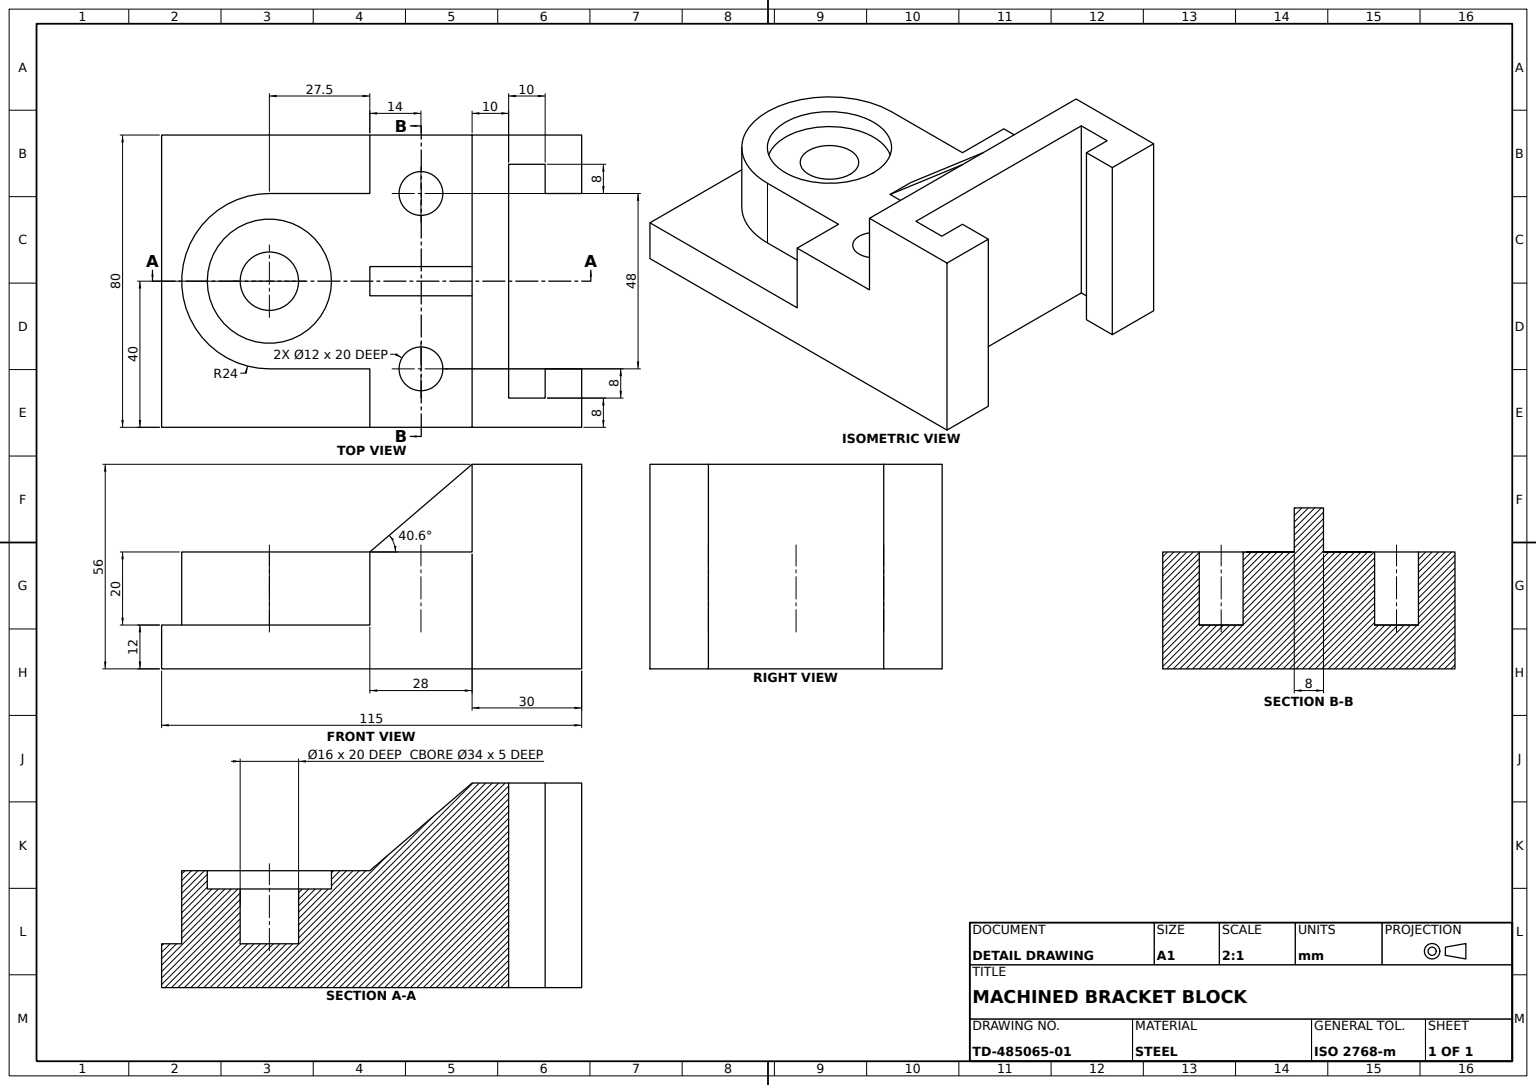
SolidWorks part; units mm, degrees
material "Plain Carbon Steel"
ref_plane "Front Plane" through (0, 0, 0) normal (0, 0, 1) x (1, 0, 0)
ref_plane "Top Plane" through (0, 0, 0) normal (0, 1, 0) x (1, 0, 0)
ref_plane "Right Plane" through (0, 0, 0) normal (1, 0, 0) x (0, 0, -1)
sketch "Base Plate Sketch" plane through (0, 0, 0) normal (0, 1, 0) x (1, 0, 0)
  line L1 (-40, -57.5) -> (40, -57.5)
  line L2 (-40, -57.5) -> (-40, 57.5)
  line L3 (-40, 57.5) -> (40, 57.5)
  line L4 (40, -57.5) -> (40, 57.5)
  line L5 (-40, -57.5) -> (40, 57.5) construction
  line L6 (-40, 57.5) -> (40, -57.5) construction
  point P0 (0, 0)
  dimension "D1" = 115
  dimension "D2" = 80
extrude "Base Plate" add sketch "Base Plate Sketch" along normal blind 12
sketch "Back Wall Sketch" plane through (0, 12, 0) normal (0, 1, 0) x (1, 0, 0)
  line L0 (40, -57.5) -> (40, 57.5) construction
  line L1 (-40, 57.5) -> (40, 57.5)
  line L2 (-40, 57.5) -> (-40, 27.5)
  line L3 (-40, 27.5) -> (40, 27.5)
  line L4 (40, 57.5) -> (40, 27.5)
  dimension "D1" = 30
extrude "Back Wall" add sketch "Back Wall Sketch" along normal blind 44
sketch "Wall Slot Sketch" plane through (0, 56, 0) normal (0, 1, 0) x (1, 0, 0)
  line L0 (-24, 57.5) -> (-24, 47.5)
  line L1 (40, 57.5) -> (-40, 57.5) construction
  line L2 (-24, 47.5) -> (-32, 47.5)
  line L3 (-32, 47.5) -> (-32, 37.5)
  line L4 (-32, 37.5) -> (32, 37.5)
  line L5 (32, 37.5) -> (32, 47.5)
  line L6 (32, 47.5) -> (24, 47.5)
  line L7 (24, 47.5) -> (24, 57.5)
  line L8 (24, 57.5) -> (-24, 57.5)
  dimension "D1" = 16
  dimension "D2" = 16
  dimension "D3" = 10
  dimension "D4" = 10
  dimension "D5" = 8
  dimension "D6" = 8
  dimension "D7" = 10
extrude "Wall Slot Cut" cut sketch "Wall Slot Sketch" against normal through all
sketch "Boss Pad Sketch" plane through (0, 12, 0) normal (0, 1, 0) x (1, 0, 0)
  line L0 (40, -57.5) -> (40, 27.5) construction
  line L1 (-40, 27.5) -> (40, 27.5)
  line L2 (-40, 27.5) -> (-40, -0.5)
  line L3 (-40, -0.5) -> (-24, -0.5)
  line L4 (40, 27.5) -> (40, -0.5)
  line L5 (-24, -28) -> (-24, -0.5)
  line L6 (24, -28) -> (24, -0.5)
  line L7 (24, -0.5) -> (40, -0.5)
  arc A0 (-24, -28) -> (24, -28) centre (0, -28) ccw
  circle A1 centre (-24, 13.5) radius 6
  circle A2 centre (24, 13.5) radius 6
  dimension "D2" = 48
  dimension "D5" = 12
  dimension "D6" = 12
  dimension "D1" = 28
  dimension "D3" = 28
  dimension "D4" = 27.5
  dimension "D7" = 14
  dimension "D8" = 16
  dimension "D9" = 14
  dimension "D10" = 16
extrude "Boss Pad" add sketch "Boss Pad Sketch" along normal blind 20
sketch "Counterbore Sketch" plane through (0, 32, 0) normal (0, 1, 0) x (1, 0, 0)
  circle A0 centre (0, -28) radius 17
  dimension "D1" = 34
extrude "Counterbore Ø34x5" cut sketch "Counterbore Sketch" against normal blind 5
sketch "Bore Sketch" plane through (0, 27, 0) normal (0, 1, 0) x (1, 0, 0)
  circle A0 centre (0, -28) radius 8
  dimension "D1" = 16
extrude "Bore Ø16" cut sketch "Bore Sketch" against normal blind 15
ref_plane "Plane2" through (0, 0, 0) normal (1, 0, 0) x (0, 0, -1)
sketch "Rib Sketch" plane through (0, 0, 0) normal (1, 0, 0) x (0, 0, -1)
  line L0 (27.5, 56) -> (-0.5, 32)
rib "Support Rib 8mm" sketch "Rib Sketch" sketch "Rib Sketch" thickness 8 extrusion direction parallel to sketch draft on no parameters "D1"=8
